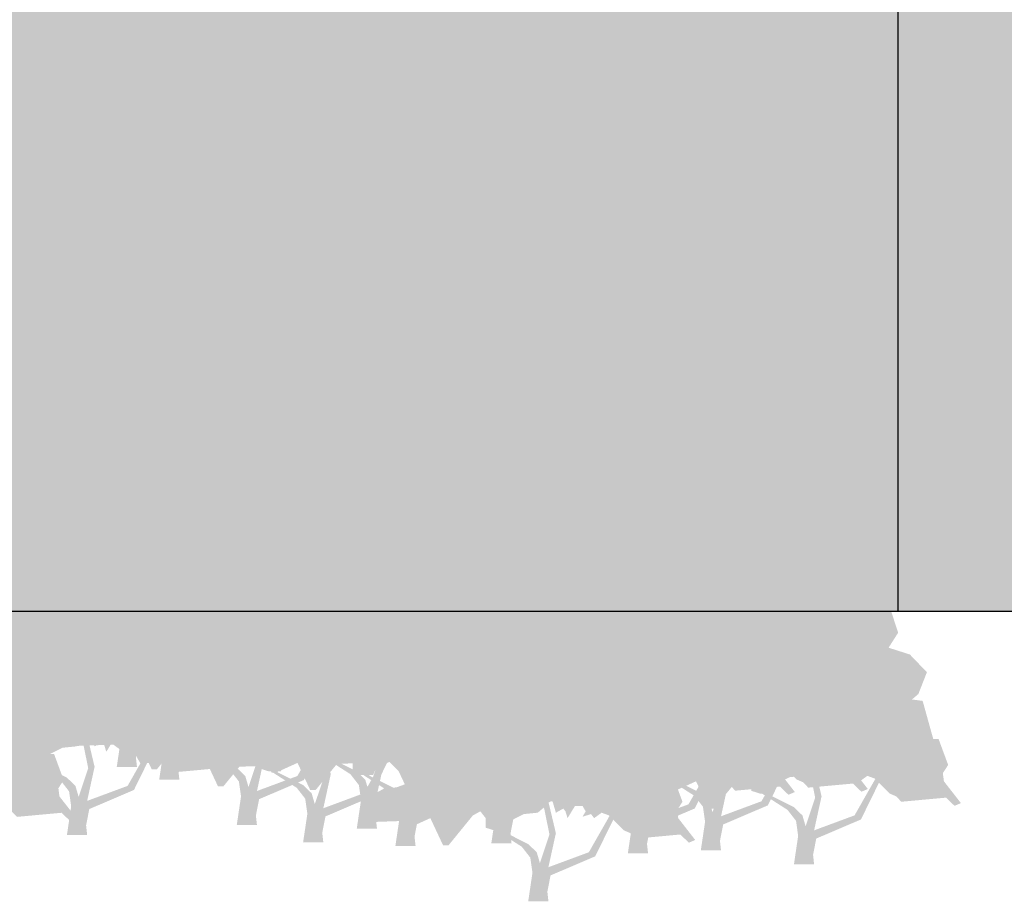
# Model space of a CAD drawing. Units: feet. Extents: x 2368 to 3224, y 836 to 1229.
# Tile 3 of 9: x 2413 to 2447, y 844 to 873. Entities that reach past the tile are written whole.
import ezdxf

# ---------------------------------------------------------------- set-up
doc = ezdxf.new("R2010")
doc.units = ezdxf.units.FT
for name, color, linetype, lineweight in [('A-ELEV', 7, 'Continuous', 25), ('A-ELEV-PATT', 8, 'Continuous', 13), ('L-PLNT', 3, 'Continuous', 13)]:
    doc.layers.add(name, color=color, linetype=linetype, lineweight=lineweight)

msp = doc.modelspace()

# ---------------------------------------------------------------- hatches: boundary and pattern name
at = {"layer": 'A-ELEV-PATT'}
h = msp.add_hatch(color=256, dxfattribs=at)
h.dxf.hatch_style = 1
h.paths.add_polyline_path([(2443.042, 973.51), (2394.909, 973.51), (2394.909, 853.51), (2443.042, 853.51)])
h.paths.add_polyline_path([(2422.205, 920.108), (2422.205, 905.784), (2416.403, 905.784), (2416.403, 920.108)], flags=16)
h.paths.add_polyline_path([(2449.299, 970.694), (2443.042, 973.51), (2443.042, 853.51), (2449.299, 853.51)])
h.paths.add_polyline_path([(2510.022, 987.861), (2368.302, 987.861), (2394.909, 973.51), (2443.042, 973.51), (2510.022, 973.51)])
h.paths.add_polyline_path([(2510.022, 973.51), (2443.042, 973.51), (2449.299, 970.694), (2510.022, 970.694)])
at = {"layer": 'L-PLNT'}
h = msp.add_hatch(color=256, dxfattribs=at)
h.dxf.hatch_style = 1
h.paths.add_polyline_path([(2428.131, 855.842), (2427.556, 856.441), (2426.837, 856.672), (2427.161, 857.179), (2426.873, 858.054), (2426.694, 858.054), (2426.334, 858.838), (2426.119, 858.791), (2425.867, 858.791), (2425.687, 859.16), (2425.795, 859.667), (2426.083, 859.667), (2425.543, 860.312), (2425.471, 860.824), (2425.184, 861.142), (2424.932, 860.865), (2424.789, 860.957), (2424.753, 861.188), (2424.573, 861.28), (2424.321, 861.049), (2424.034, 861.096), (2423.818, 860.681), (2423.818, 860.312), (2424.106, 860.174), (2423.89, 860.036), (2423.674, 860.22), (2423.063, 859.621), (2423.063, 859.483), (2422.812, 859.344), (2422.883, 859.206), (2423.063, 858.93), (2422.74, 858.699), (2422.416, 858.93), (2422.236, 858.884), (2422.165, 858.699), (2422.416, 858.653), (2422.452, 858.285), (2422.171, 858.331), (2421.841, 858.008), (2422.201, 857.962), (2422.057, 857.501), (2421.733, 857.455), (2421.374, 857.225), (2420.942, 856.994), (2420.907, 857.179), (2420.583, 856.487), (2421.158, 856.626), (2421.518, 856.395), (2421.41, 855.842), (2420.763, 855.612), (2420.475, 855.796), (2420.367, 855.52), (2420.116, 855.474), (2419.9, 855.197), (2419.648, 854.875), (2419.972, 854.598), (2420.188, 854.736), (2419.944, 854.336), (2420.121, 854.356), (2420.095, 853.994), (2419.505, 853.216), (2418.786, 853.17), (2418.462, 852.985), (2417.923, 852.386), (2418.139, 852.017), (2419.469, 852.064), (2419.72, 851.879), (2420.331, 852.156), (2420.763, 851.234), (2420.942, 851.234), (2421.769, 852.248), (2422.021, 852.386), (2422.201, 852.156), (2422.201, 851.833), (2422.488, 851.741), (2422.883, 851.741), (2423.027, 852.064), (2423.495, 852.294), (2423.962, 852.34), (2424.178, 852.524), (2424.213, 852.57), (2424.321, 852.801), (2424.465, 852.709), (2424.573, 852.34), (2424.825, 852.478), (2424.896, 852.386), (2424.968, 852.156), (2425.22, 852.57), (2425.472, 852.57), (2425.579, 852.386), (2425.472, 852.202), (2425.759, 852.294), (2425.867, 852.156), (2426.119, 852.34), (2426.37, 852.248), (2426.873, 851.741), (2427.089, 851.649), (2427.269, 851.465), (2428.778, 851.603), (2429.066, 851.326), (2429.282, 851.418), (2428.707, 852.156), (2428.671, 852.432), (2428.85, 852.709), (2428.527, 853.584), (2428.347, 853.584), (2427.988, 854.875), (2427.628, 854.921), (2427.844, 855.105)])
h = msp.add_hatch(color=256, dxfattribs=at)
h.dxf.hatch_style = 1
h.paths.add_polyline_path([(2414.456, 854.681), (2413.881, 855.281), (2413.162, 855.511), (2413.485, 856.018), (2413.198, 856.893), (2413.018, 856.893), (2412.659, 857.677), (2412.443, 857.631), (2412.191, 857.631), (2412.012, 857.999), (2412.12, 858.506), (2412.407, 858.506), (2411.868, 859.151), (2411.795, 859.663), (2411.509, 859.981), (2411.257, 859.704), (2411.113, 859.797), (2411.077, 860.027), (2410.897, 860.119), (2410.646, 859.889), (2410.358, 859.935), (2410.143, 859.52), (2410.143, 859.151), (2410.43, 859.013), (2410.214, 858.875), (2409.999, 859.059), (2409.388, 858.46), (2409.388, 858.322), (2409.136, 858.184), (2409.208, 858.045), (2409.388, 857.769), (2409.064, 857.539), (2408.741, 857.769), (2408.561, 857.723), (2408.489, 857.539), (2408.741, 857.492), (2408.777, 857.124), (2408.496, 857.17), (2408.166, 856.847), (2408.525, 856.801), (2408.381, 856.34), (2408.058, 856.294), (2407.698, 856.064), (2407.267, 855.834), (2407.231, 856.018), (2406.908, 855.327), (2407.483, 855.465), (2407.842, 855.234), (2407.734, 854.681), (2407.087, 854.451), (2406.8, 854.635), (2406.692, 854.359), (2406.44, 854.313), (2406.225, 854.036), (2405.973, 853.714), (2406.297, 853.437), (2406.512, 853.576), (2406.268, 853.175), (2406.445, 853.195), (2406.42, 852.833), (2405.829, 852.055), (2405.11, 852.009), (2404.787, 851.824), (2404.248, 851.225), (2404.463, 850.857), (2405.793, 850.903), (2406.045, 850.718), (2406.656, 850.995), (2407.087, 850.073), (2407.267, 850.073), (2408.094, 851.087), (2408.345, 851.225), (2408.525, 850.995), (2408.525, 850.672), (2408.813, 850.58), (2409.208, 850.58), (2409.352, 850.903), (2409.819, 851.133), (2410.286, 851.179), (2410.502, 851.364), (2410.538, 851.41), (2410.646, 851.64), (2410.79, 851.548), (2410.897, 851.179), (2411.149, 851.318), (2411.221, 851.225), (2411.293, 850.995), (2411.544, 851.41), (2411.796, 851.41), (2411.904, 851.225), (2411.796, 851.041), (2412.084, 851.133), (2412.191, 850.995), (2412.443, 851.179), (2412.695, 851.087), (2413.198, 850.58), (2413.414, 850.488), (2413.593, 850.304), (2415.103, 850.442), (2415.391, 850.165), (2415.606, 850.258), (2415.031, 850.995), (2414.995, 851.271), (2415.175, 851.548), (2414.851, 852.423), (2414.672, 852.423), (2414.312, 853.714), (2413.953, 853.76), (2414.168, 853.944)])
h = msp.add_hatch(color=256, dxfattribs=at)
h.dxf.hatch_style = 1
h.paths.add_polyline_path([(2421.127, 854.737), (2420.552, 855.336), (2419.833, 855.567), (2420.157, 856.074), (2419.869, 856.949), (2419.689, 856.949), (2419.33, 857.732), (2419.114, 857.686), (2418.862, 857.686), (2418.683, 858.055), (2418.791, 858.562), (2419.078, 858.562), (2418.539, 859.207), (2418.466, 859.718), (2418.18, 860.037), (2417.928, 859.76), (2417.784, 859.852), (2417.748, 860.083), (2417.568, 860.175), (2417.317, 859.944), (2417.029, 859.99), (2416.814, 859.576), (2416.814, 859.207), (2417.101, 859.069), (2416.886, 858.931), (2416.67, 859.115), (2416.059, 858.516), (2416.059, 858.378), (2415.807, 858.239), (2415.879, 858.101), (2416.059, 857.825), (2415.735, 857.594), (2415.412, 857.825), (2415.232, 857.779), (2415.16, 857.594), (2415.412, 857.548), (2415.448, 857.179), (2415.167, 857.226), (2414.837, 856.903), (2415.196, 856.857), (2415.052, 856.396), (2414.729, 856.35), (2414.369, 856.12), (2413.938, 855.889), (2413.902, 856.074), (2413.579, 855.382), (2414.154, 855.521), (2414.513, 855.29), (2414.405, 854.737), (2413.758, 854.507), (2413.471, 854.691), (2413.363, 854.415), (2413.111, 854.369), (2412.896, 854.092), (2412.644, 853.769), (2412.968, 853.493), (2413.183, 853.631), (2412.939, 853.23), (2413.117, 853.251), (2413.091, 852.888), (2412.5, 852.111), (2411.781, 852.064), (2411.458, 851.88), (2410.919, 851.281), (2411.134, 850.912), (2412.464, 850.958), (2412.716, 850.774), (2413.327, 851.051), (2413.758, 850.129), (2413.938, 850.129), (2414.765, 851.143), (2415.016, 851.281), (2415.196, 851.051), (2415.196, 850.728), (2415.484, 850.636), (2415.879, 850.636), (2416.023, 850.958), (2416.49, 851.189), (2416.957, 851.235), (2417.173, 851.419), (2417.209, 851.465), (2417.317, 851.696), (2417.461, 851.604), (2417.568, 851.235), (2417.82, 851.373), (2417.892, 851.281), (2417.964, 851.051), (2418.215, 851.465), (2418.467, 851.465), (2418.575, 851.281), (2418.467, 851.097), (2418.755, 851.189), (2418.862, 851.051), (2419.114, 851.235), (2419.366, 851.143), (2419.869, 850.636), (2420.085, 850.544), (2420.264, 850.359), (2421.774, 850.498), (2422.062, 850.221), (2422.277, 850.313), (2421.702, 851.051), (2421.666, 851.327), (2421.846, 851.604), (2421.522, 852.479), (2421.343, 852.479), (2420.983, 853.769), (2420.624, 853.816), (2420.839, 854)])
h = msp.add_hatch(color=256, dxfattribs=at)
h.dxf.hatch_style = 1
h.paths.add_polyline_path([(2422.561, 854.308), (2421.986, 854.907), (2421.267, 855.137), (2421.591, 855.644), (2421.303, 856.52), (2421.123, 856.52), (2420.764, 857.303), (2420.548, 857.257), (2420.297, 857.257), (2420.117, 857.626), (2420.225, 858.132), (2420.512, 858.132), (2419.973, 858.778), (2419.901, 859.289), (2419.614, 859.607), (2419.362, 859.331), (2419.218, 859.423), (2419.182, 859.653), (2419.003, 859.745), (2418.751, 859.515), (2418.463, 859.561), (2418.248, 859.146), (2418.248, 858.778), (2418.535, 858.639), (2418.32, 858.501), (2418.104, 858.685), (2417.493, 858.086), (2417.493, 857.948), (2417.241, 857.81), (2417.313, 857.672), (2417.493, 857.395), (2417.169, 857.165), (2416.846, 857.395), (2416.666, 857.349), (2416.594, 857.165), (2416.846, 857.119), (2416.882, 856.75), (2416.601, 856.796), (2416.271, 856.474), (2416.63, 856.427), (2416.486, 855.967), (2416.163, 855.921), (2415.804, 855.69), (2415.372, 855.46), (2415.336, 855.644), (2415.013, 854.953), (2415.588, 855.091), (2415.947, 854.861), (2415.839, 854.308), (2415.192, 854.077), (2414.905, 854.262), (2414.797, 853.985), (2414.545, 853.939), (2414.33, 853.663), (2414.078, 853.34), (2414.402, 853.063), (2414.617, 853.202), (2414.374, 852.801), (2414.551, 852.822), (2414.525, 852.459), (2413.934, 851.681), (2413.215, 851.635), (2412.892, 851.451), (2412.353, 850.852), (2412.568, 850.483), (2413.898, 850.529), (2414.15, 850.345), (2414.761, 850.621), (2415.192, 849.7), (2415.372, 849.7), (2416.199, 850.713), (2416.451, 850.852), (2416.63, 850.621), (2416.63, 850.299), (2416.918, 850.206), (2417.313, 850.206), (2417.457, 850.529), (2417.924, 850.759), (2418.392, 850.806), (2418.607, 850.99), (2418.643, 851.036), (2418.751, 851.266), (2418.895, 851.174), (2419.003, 850.806), (2419.254, 850.944), (2419.326, 850.852), (2419.398, 850.621), (2419.65, 851.036), (2419.901, 851.036), (2420.009, 850.852), (2419.901, 850.667), (2420.189, 850.759), (2420.297, 850.621), (2420.548, 850.806), (2420.8, 850.713), (2421.303, 850.206), (2421.519, 850.114), (2421.698, 849.93), (2423.208, 850.068), (2423.496, 849.792), (2423.711, 849.884), (2423.136, 850.621), (2423.1, 850.898), (2423.28, 851.174), (2422.957, 852.05), (2422.777, 852.05), (2422.417, 853.34), (2422.058, 853.386), (2422.274, 853.57)])
h = msp.add_hatch(color=256, dxfattribs=at)
h.dxf.hatch_style = 1
h.paths.add_polyline_path([(2425.182, 852.773), (2424.607, 853.372), (2423.888, 853.602), (2424.212, 854.109), (2423.924, 854.985), (2423.744, 854.985), (2423.385, 855.768), (2423.169, 855.722), (2422.918, 855.722), (2422.738, 856.09), (2422.846, 856.597), (2423.133, 856.597), (2422.594, 857.242), (2422.522, 857.754), (2422.235, 858.072), (2421.983, 857.795), (2421.839, 857.888), (2421.803, 858.118), (2421.624, 858.21), (2421.372, 857.98), (2421.085, 858.026), (2420.869, 857.611), (2420.869, 857.242), (2421.156, 857.104), (2420.941, 856.966), (2420.725, 857.15), (2420.114, 856.551), (2420.114, 856.413), (2419.862, 856.275), (2419.934, 856.137), (2420.114, 855.86), (2419.79, 855.63), (2419.467, 855.86), (2419.287, 855.814), (2419.215, 855.63), (2419.467, 855.584), (2419.503, 855.215), (2419.222, 855.261), (2418.892, 854.938), (2419.251, 854.892), (2419.108, 854.432), (2418.784, 854.385), (2418.425, 854.155), (2417.993, 853.925), (2417.957, 854.109), (2417.634, 853.418), (2418.209, 853.556), (2418.568, 853.326), (2418.461, 852.773), (2417.814, 852.542), (2417.526, 852.727), (2417.418, 852.45), (2417.167, 852.404), (2416.951, 852.127), (2416.699, 851.805), (2417.023, 851.528), (2417.238, 851.667), (2416.995, 851.266), (2417.172, 851.287), (2417.146, 850.924), (2416.555, 850.146), (2415.837, 850.1), (2415.513, 849.916), (2414.974, 849.316), (2415.19, 848.948), (2416.52, 848.994), (2416.771, 848.81), (2417.382, 849.086), (2417.814, 848.164), (2417.993, 848.164), (2418.82, 849.178), (2419.072, 849.316), (2419.251, 849.086), (2419.251, 848.763), (2419.539, 848.671), (2419.934, 848.671), (2420.078, 848.994), (2420.545, 849.224), (2421.013, 849.27), (2421.228, 849.455), (2421.264, 849.501), (2421.372, 849.731), (2421.516, 849.639), (2421.624, 849.27), (2421.875, 849.409), (2421.947, 849.316), (2422.019, 849.086), (2422.271, 849.501), (2422.522, 849.501), (2422.63, 849.316), (2422.522, 849.132), (2422.81, 849.224), (2422.918, 849.086), (2423.169, 849.27), (2423.421, 849.178), (2423.924, 848.671), (2424.14, 848.579), (2424.32, 848.395), (2425.829, 848.533), (2426.117, 848.257), (2426.332, 848.349), (2425.757, 849.086), (2425.721, 849.363), (2425.901, 849.639), (2425.578, 850.515), (2425.398, 850.515), (2425.038, 851.805), (2424.679, 851.851), (2424.895, 852.035)])
h = msp.add_hatch(color=256, dxfattribs=at)
h.dxf.hatch_style = 1
h.paths.add_polyline_path([(2429.237, 852.65), (2428.662, 853.249), (2427.943, 853.479), (2428.267, 853.986), (2427.979, 854.862), (2427.8, 854.862), (2427.44, 855.645), (2427.224, 855.599), (2426.973, 855.599), (2426.793, 855.968), (2426.901, 856.475), (2427.189, 856.475), (2426.649, 857.12), (2426.577, 857.631), (2426.29, 857.949), (2426.038, 857.673), (2425.895, 857.765), (2425.859, 857.995), (2425.679, 858.087), (2425.427, 857.857), (2425.14, 857.903), (2424.924, 857.488), (2424.924, 857.12), (2425.212, 856.981), (2424.996, 856.843), (2424.78, 857.028), (2424.169, 856.428), (2424.169, 856.29), (2423.918, 856.152), (2423.989, 856.014), (2424.169, 855.737), (2423.846, 855.507), (2423.522, 855.737), (2423.342, 855.691), (2423.271, 855.507), (2423.522, 855.461), (2423.558, 855.092), (2423.277, 855.138), (2422.947, 854.816), (2423.307, 854.77), (2423.163, 854.309), (2422.839, 854.263), (2422.48, 854.032), (2422.048, 853.802), (2422.012, 853.986), (2421.689, 853.295), (2422.264, 853.433), (2422.624, 853.203), (2422.516, 852.65), (2421.869, 852.419), (2421.581, 852.604), (2421.473, 852.327), (2421.222, 852.281), (2421.006, 852.005), (2420.754, 851.682), (2421.078, 851.406), (2421.294, 851.544), (2421.05, 851.143), (2421.227, 851.164), (2421.201, 850.801), (2420.611, 850.023), (2419.892, 849.977), (2419.568, 849.793), (2419.029, 849.194), (2419.245, 848.825), (2420.575, 848.871), (2420.826, 848.687), (2421.437, 848.963), (2421.869, 848.042), (2422.048, 848.042), (2422.875, 849.055), (2423.127, 849.194), (2423.307, 848.963), (2423.307, 848.641), (2423.594, 848.549), (2423.989, 848.549), (2424.133, 848.871), (2424.601, 849.102), (2425.068, 849.148), (2425.283, 849.332), (2425.319, 849.378), (2425.427, 849.608), (2425.571, 849.516), (2425.679, 849.148), (2425.93, 849.286), (2426.002, 849.194), (2426.074, 848.963), (2426.326, 849.378), (2426.577, 849.378), (2426.685, 849.194), (2426.577, 849.009), (2426.865, 849.102), (2426.973, 848.963), (2427.224, 849.148), (2427.476, 849.055), (2427.979, 848.549), (2428.195, 848.456), (2428.375, 848.272), (2429.884, 848.41), (2430.172, 848.134), (2430.388, 848.226), (2429.813, 848.963), (2429.777, 849.24), (2429.956, 849.516), (2429.633, 850.392), (2429.453, 850.392), (2429.094, 851.682), (2428.734, 851.728), (2428.95, 851.912)])
h = msp.add_hatch(color=256, dxfattribs=at)
h.dxf.hatch_style = 1
h.paths.add_polyline_path([(2419.444, 852.439), (2418.869, 853.038), (2418.15, 853.268), (2418.473, 853.775), (2418.186, 854.651), (2418.006, 854.651), (2417.647, 855.434), (2417.431, 855.388), (2417.179, 855.388), (2417, 855.757), (2417.107, 856.264), (2417.395, 856.264), (2416.856, 856.909), (2416.783, 857.42), (2416.496, 857.738), (2416.245, 857.462), (2416.101, 857.554), (2416.065, 857.784), (2415.885, 857.876), (2415.634, 857.646), (2415.346, 857.692), (2415.13, 857.277), (2415.13, 856.909), (2415.418, 856.77), (2415.202, 856.632), (2414.987, 856.817), (2414.376, 856.217), (2414.376, 856.079), (2414.124, 855.941), (2414.196, 855.803), (2414.376, 855.526), (2414.052, 855.296), (2413.729, 855.526), (2413.549, 855.48), (2413.477, 855.296), (2413.729, 855.25), (2413.764, 854.881), (2413.483, 854.927), (2413.153, 854.605), (2413.513, 854.559), (2413.369, 854.098), (2413.046, 854.052), (2412.686, 853.821), (2412.255, 853.591), (2412.219, 853.775), (2411.895, 853.084), (2412.47, 853.222), (2412.83, 852.992), (2412.722, 852.439), (2412.075, 852.208), (2411.788, 852.393), (2411.68, 852.116), (2411.428, 852.07), (2411.212, 851.794), (2410.961, 851.471), (2411.284, 851.195), (2411.5, 851.333), (2411.256, 850.932), (2411.433, 850.953), (2411.408, 850.59), (2410.817, 849.812), (2410.098, 849.766), (2409.775, 849.582), (2409.235, 848.983), (2409.451, 848.614), (2410.781, 848.66), (2411.033, 848.476), (2411.644, 848.752), (2412.075, 847.831), (2412.255, 847.831), (2413.082, 848.844), (2413.333, 848.983), (2413.513, 848.752), (2413.513, 848.43), (2413.8, 848.338), (2414.196, 848.338), (2414.34, 848.66), (2414.807, 848.89), (2415.274, 848.937), (2415.49, 849.121), (2415.526, 849.167), (2415.634, 849.397), (2415.777, 849.305), (2415.885, 848.937), (2416.137, 849.075), (2416.209, 848.983), (2416.281, 848.752), (2416.532, 849.167), (2416.784, 849.167), (2416.892, 848.983), (2416.784, 848.798), (2417.071, 848.89), (2417.179, 848.752), (2417.431, 848.937), (2417.682, 848.844), (2418.186, 848.338), (2418.401, 848.245), (2418.581, 848.061), (2420.091, 848.199), (2420.378, 847.923), (2420.594, 848.015), (2420.019, 848.752), (2419.983, 849.029), (2420.163, 849.305), (2419.839, 850.181), (2419.659, 850.181), (2419.3, 851.471), (2418.941, 851.517), (2419.156, 851.701)])
h = msp.add_hatch(color=256, dxfattribs=at)
h.dxf.hatch_style = 1
h.paths.add_polyline_path([(2427.424, 852.19), (2426.849, 852.789), (2426.13, 853.019), (2426.454, 853.526), (2426.166, 854.401), (2425.986, 854.401), (2425.627, 855.185), (2425.411, 855.139), (2425.16, 855.139), (2424.98, 855.507), (2425.088, 856.014), (2425.375, 856.014), (2424.836, 856.659), (2424.764, 857.171), (2424.477, 857.489), (2424.225, 857.212), (2424.081, 857.305), (2424.045, 857.535), (2423.866, 857.627), (2423.614, 857.397), (2423.327, 857.443), (2423.111, 857.028), (2423.111, 856.659), (2423.398, 856.521), (2423.183, 856.383), (2422.967, 856.567), (2422.356, 855.968), (2422.356, 855.83), (2422.104, 855.692), (2422.176, 855.554), (2422.356, 855.277), (2422.033, 855.047), (2421.709, 855.277), (2421.529, 855.231), (2421.457, 855.047), (2421.709, 855.001), (2421.745, 854.632), (2421.464, 854.678), (2421.134, 854.355), (2421.493, 854.309), (2421.35, 853.849), (2421.026, 853.802), (2420.667, 853.572), (2420.235, 853.342), (2420.199, 853.526), (2419.876, 852.835), (2420.451, 852.973), (2420.81, 852.743), (2420.703, 852.19), (2420.056, 851.959), (2419.768, 852.143), (2419.66, 851.867), (2419.409, 851.821), (2419.193, 851.544), (2418.941, 851.222), (2419.265, 850.945), (2419.48, 851.084), (2419.237, 850.683), (2419.414, 850.704), (2419.388, 850.341), (2418.797, 849.563), (2418.079, 849.517), (2417.755, 849.333), (2417.216, 848.733), (2417.432, 848.365), (2418.762, 848.411), (2419.013, 848.227), (2419.624, 848.503), (2420.056, 847.581), (2420.235, 847.581), (2421.062, 848.595), (2421.314, 848.733), (2421.493, 848.503), (2421.493, 848.18), (2421.781, 848.088), (2422.176, 848.088), (2422.32, 848.411), (2422.787, 848.641), (2423.255, 848.687), (2423.47, 848.872), (2423.506, 848.918), (2423.614, 849.148), (2423.758, 849.056), (2423.866, 848.687), (2424.117, 848.826), (2424.189, 848.733), (2424.261, 848.503), (2424.513, 848.918), (2424.764, 848.918), (2424.872, 848.733), (2424.764, 848.549), (2425.052, 848.641), (2425.16, 848.503), (2425.411, 848.687), (2425.663, 848.595), (2426.166, 848.088), (2426.382, 847.996), (2426.562, 847.812), (2428.071, 847.95), (2428.359, 847.674), (2428.574, 847.766), (2427.999, 848.503), (2427.963, 848.78), (2428.143, 849.056), (2427.82, 849.932), (2427.64, 849.932), (2427.28, 851.222), (2426.921, 851.268), (2427.137, 851.452)])
h = msp.add_hatch(color=256, dxfattribs=at)
h.dxf.hatch_style = 1
h.paths.add_polyline_path([(2430.542, 852.065), (2429.966, 852.664), (2429.248, 852.894), (2429.571, 853.401), (2429.284, 854.277), (2429.104, 854.277), (2428.744, 855.06), (2428.529, 855.014), (2428.277, 855.014), (2428.097, 855.383), (2428.205, 855.89), (2428.493, 855.89), (2427.954, 856.535), (2427.881, 857.046), (2427.594, 857.364), (2427.343, 857.088), (2427.199, 857.18), (2427.163, 857.41), (2426.983, 857.503), (2426.731, 857.272), (2426.444, 857.318), (2426.228, 856.904), (2426.228, 856.535), (2426.516, 856.397), (2426.3, 856.258), (2426.084, 856.443), (2425.473, 855.844), (2425.473, 855.705), (2425.222, 855.567), (2425.294, 855.429), (2425.473, 855.152), (2425.15, 854.922), (2424.826, 855.152), (2424.647, 855.106), (2424.575, 854.922), (2424.826, 854.876), (2424.862, 854.507), (2424.581, 854.553), (2424.251, 854.231), (2424.611, 854.185), (2424.467, 853.724), (2424.143, 853.678), (2423.784, 853.447), (2423.353, 853.217), (2423.317, 853.401), (2422.993, 852.71), (2423.568, 852.848), (2423.928, 852.618), (2423.82, 852.065), (2423.173, 851.835), (2422.885, 852.019), (2422.778, 851.742), (2422.526, 851.696), (2422.31, 851.42), (2422.059, 851.097), (2422.382, 850.821), (2422.598, 850.959), (2422.354, 850.558), (2422.531, 850.579), (2422.506, 850.216), (2421.915, 849.438), (2421.196, 849.392), (2420.872, 849.208), (2420.333, 848.609), (2420.549, 848.24), (2421.879, 848.286), (2422.131, 848.102), (2422.742, 848.378), (2423.173, 847.457), (2423.353, 847.457), (2424.179, 848.471), (2424.431, 848.609), (2424.611, 848.378), (2424.611, 848.056), (2424.898, 847.964), (2425.294, 847.964), (2425.437, 848.286), (2425.905, 848.517), (2426.372, 848.563), (2426.588, 848.747), (2426.624, 848.793), (2426.731, 849.024), (2426.875, 848.931), (2426.983, 848.563), (2427.235, 848.701), (2427.307, 848.609), (2427.378, 848.378), (2427.63, 848.793), (2427.882, 848.793), (2427.99, 848.609), (2427.882, 848.425), (2428.169, 848.517), (2428.277, 848.378), (2428.529, 848.563), (2428.78, 848.471), (2429.284, 847.964), (2429.499, 847.872), (2429.679, 847.687), (2431.189, 847.825), (2431.476, 847.549), (2431.692, 847.641), (2431.117, 848.378), (2431.081, 848.655), (2431.261, 848.931), (2430.937, 849.807), (2430.757, 849.807), (2430.398, 851.097), (2430.038, 851.143), (2430.254, 851.328)])
h = msp.add_hatch(color=256, dxfattribs=at)
h.dxf.hatch_style = 1
h.paths.add_polyline_path([(2433.784, 852.159), (2433.209, 852.758), (2432.49, 852.988), (2432.814, 853.495), (2432.526, 854.371), (2432.346, 854.371), (2431.987, 855.154), (2431.771, 855.108), (2431.52, 855.108), (2431.34, 855.477), (2431.448, 855.983), (2431.735, 855.983), (2431.196, 856.629), (2431.124, 857.14), (2430.837, 857.458), (2430.585, 857.182), (2430.441, 857.274), (2430.405, 857.504), (2430.226, 857.596), (2429.974, 857.366), (2429.686, 857.412), (2429.471, 856.997), (2429.471, 856.629), (2429.758, 856.49), (2429.543, 856.352), (2429.327, 856.536), (2428.716, 855.937), (2428.716, 855.799), (2428.464, 855.661), (2428.536, 855.523), (2428.716, 855.246), (2428.392, 855.016), (2428.069, 855.246), (2427.889, 855.2), (2427.817, 855.016), (2428.069, 854.97), (2428.105, 854.601), (2427.824, 854.647), (2427.494, 854.324), (2427.853, 854.278), (2427.709, 853.818), (2427.386, 853.772), (2427.027, 853.541), (2426.595, 853.311), (2426.559, 853.495), (2426.236, 852.804), (2426.811, 852.942), (2427.17, 852.712), (2427.062, 852.159), (2426.415, 851.928), (2426.128, 852.113), (2426.02, 851.836), (2425.768, 851.79), (2425.553, 851.514), (2425.301, 851.191), (2425.625, 850.914), (2425.84, 851.053), (2425.596, 850.652), (2425.774, 850.673), (2425.748, 850.31), (2425.157, 849.532), (2424.438, 849.486), (2424.115, 849.302), (2423.576, 848.703), (2423.791, 848.334), (2425.121, 848.38), (2425.373, 848.196), (2425.984, 848.472), (2426.415, 847.551), (2426.595, 847.551), (2427.422, 848.564), (2427.674, 848.703), (2427.853, 848.472), (2427.853, 848.15), (2428.141, 848.057), (2428.536, 848.057), (2428.68, 848.38), (2429.147, 848.61), (2429.615, 848.656), (2429.83, 848.841), (2429.866, 848.887), (2429.974, 849.117), (2430.118, 849.025), (2430.226, 848.656), (2430.477, 848.795), (2430.549, 848.703), (2430.621, 848.472), (2430.873, 848.887), (2431.124, 848.887), (2431.232, 848.703), (2431.124, 848.518), (2431.412, 848.61), (2431.52, 848.472), (2431.771, 848.656), (2432.023, 848.564), (2432.526, 848.057), (2432.742, 847.965), (2432.921, 847.781), (2434.431, 847.919), (2434.719, 847.643), (2434.934, 847.735), (2434.359, 848.472), (2434.323, 848.749), (2434.503, 849.025), (2434.18, 849.901), (2434, 849.901), (2433.64, 851.191), (2433.281, 851.237), (2433.497, 851.421)])
h = msp.add_hatch(color=256, dxfattribs=at)
h.dxf.hatch_style = 1
h.paths.add_polyline_path([(2438.397, 851.816), (2437.822, 852.415), (2437.103, 852.645), (2437.427, 853.152), (2437.139, 854.028), (2436.96, 854.028), (2436.6, 854.811), (2436.384, 854.765), (2436.133, 854.765), (2435.953, 855.134), (2436.061, 855.641), (2436.349, 855.641), (2435.809, 856.286), (2435.737, 856.797), (2435.45, 857.115), (2435.198, 856.839), (2435.055, 856.931), (2435.019, 857.161), (2434.839, 857.253), (2434.587, 857.023), (2434.3, 857.069), (2434.084, 856.654), (2434.084, 856.286), (2434.372, 856.147), (2434.156, 856.009), (2433.94, 856.194), (2433.329, 855.594), (2433.329, 855.456), (2433.078, 855.318), (2433.149, 855.18), (2433.329, 854.903), (2433.006, 854.673), (2432.682, 854.903), (2432.502, 854.857), (2432.431, 854.673), (2432.682, 854.627), (2432.718, 854.258), (2432.437, 854.304), (2432.107, 853.982), (2432.466, 853.936), (2432.323, 853.475), (2431.999, 853.429), (2431.64, 853.198), (2431.208, 852.968), (2431.172, 853.152), (2430.849, 852.461), (2431.424, 852.599), (2431.784, 852.369), (2431.676, 851.816), (2431.029, 851.585), (2430.741, 851.77), (2430.633, 851.493), (2430.382, 851.447), (2430.166, 851.171), (2429.914, 850.848), (2430.238, 850.572), (2430.454, 850.71), (2430.21, 850.309), (2430.387, 850.33), (2430.361, 849.967), (2429.771, 849.189), (2429.052, 849.143), (2428.728, 848.959), (2428.189, 848.36), (2428.405, 847.991), (2429.735, 848.037), (2429.986, 847.853), (2430.597, 848.129), (2431.029, 847.208), (2431.208, 847.208), (2432.035, 848.221), (2432.287, 848.36), (2432.466, 848.129), (2432.466, 847.807), (2432.754, 847.715), (2433.149, 847.715), (2433.293, 848.037), (2433.761, 848.268), (2434.228, 848.314), (2434.443, 848.498), (2434.479, 848.544), (2434.587, 848.774), (2434.731, 848.682), (2434.839, 848.314), (2435.09, 848.452), (2435.162, 848.36), (2435.234, 848.129), (2435.486, 848.544), (2435.737, 848.544), (2435.845, 848.36), (2435.737, 848.175), (2436.025, 848.268), (2436.133, 848.129), (2436.384, 848.314), (2436.636, 848.221), (2437.139, 847.715), (2437.355, 847.622), (2437.535, 847.438), (2439.044, 847.576), (2439.332, 847.3), (2439.548, 847.392), (2438.973, 848.129), (2438.937, 848.406), (2439.116, 848.682), (2438.793, 849.558), (2438.613, 849.558), (2438.254, 850.848), (2437.894, 850.894), (2438.11, 851.078)])
h = msp.add_hatch(color=256, dxfattribs=at)
h.dxf.hatch_style = 1
h.paths.add_polyline_path([(2440.863, 851.918), (2440.288, 852.517), (2439.569, 852.748), (2439.893, 853.255), (2439.605, 854.13), (2439.425, 854.13), (2439.066, 854.914), (2438.85, 854.868), (2438.599, 854.868), (2438.419, 855.236), (2438.527, 855.743), (2438.814, 855.743), (2438.275, 856.388), (2438.203, 856.9), (2437.916, 857.218), (2437.664, 856.941), (2437.52, 857.033), (2437.484, 857.264), (2437.305, 857.356), (2437.053, 857.126), (2436.766, 857.172), (2436.55, 856.757), (2436.55, 856.388), (2436.837, 856.25), (2436.622, 856.112), (2436.406, 856.296), (2435.795, 855.697), (2435.795, 855.559), (2435.543, 855.421), (2435.615, 855.282), (2435.795, 855.006), (2435.472, 854.775), (2435.148, 855.006), (2434.968, 854.96), (2434.896, 854.775), (2435.148, 854.729), (2435.184, 854.361), (2434.903, 854.407), (2434.573, 854.084), (2434.932, 854.038), (2434.789, 853.577), (2434.465, 853.531), (2434.106, 853.301), (2433.674, 853.07), (2433.638, 853.255), (2433.315, 852.564), (2433.89, 852.702), (2434.249, 852.471), (2434.142, 851.918), (2433.495, 851.688), (2433.207, 851.872), (2433.099, 851.596), (2432.848, 851.55), (2432.632, 851.273), (2432.38, 850.951), (2432.704, 850.674), (2432.919, 850.812), (2432.676, 850.412), (2432.853, 850.432), (2432.827, 850.07), (2432.237, 849.292), (2431.518, 849.246), (2431.194, 849.061), (2430.655, 848.462), (2430.871, 848.094), (2432.201, 848.14), (2432.452, 847.955), (2433.063, 848.232), (2433.495, 847.31), (2433.674, 847.31), (2434.501, 848.324), (2434.753, 848.462), (2434.932, 848.232), (2434.932, 847.909), (2435.22, 847.817), (2435.615, 847.817), (2435.759, 848.14), (2436.226, 848.37), (2436.694, 848.416), (2436.909, 848.601), (2436.945, 848.647), (2437.053, 848.877), (2437.197, 848.785), (2437.305, 848.416), (2437.556, 848.554), (2437.628, 848.462), (2437.7, 848.232), (2437.952, 848.647), (2438.203, 848.647), (2438.311, 848.462), (2438.203, 848.278), (2438.491, 848.37), (2438.599, 848.232), (2438.85, 848.416), (2439.102, 848.324), (2439.605, 847.817), (2439.821, 847.725), (2440.001, 847.541), (2441.51, 847.679), (2441.798, 847.402), (2442.014, 847.495), (2441.438, 848.232), (2441.402, 848.508), (2441.582, 848.785), (2441.259, 849.66), (2441.079, 849.66), (2440.719, 850.951), (2440.36, 850.997), (2440.576, 851.181)])
h = msp.add_hatch(color=256, dxfattribs=at)
h.dxf.hatch_style = 1
h.paths.add_polyline_path([(2444.009, 851.442), (2443.434, 852.041), (2442.715, 852.271), (2443.038, 852.778), (2442.751, 853.654), (2442.571, 853.654), (2442.211, 854.437), (2441.996, 854.391), (2441.744, 854.391), (2441.564, 854.76), (2441.672, 855.267), (2441.96, 855.267), (2441.421, 855.912), (2441.348, 856.423), (2441.061, 856.741), (2440.81, 856.465), (2440.666, 856.557), (2440.63, 856.787), (2440.45, 856.88), (2440.198, 856.649), (2439.911, 856.695), (2439.695, 856.281), (2439.695, 855.912), (2439.983, 855.774), (2439.767, 855.635), (2439.551, 855.82), (2438.94, 855.221), (2438.94, 855.082), (2438.689, 854.944), (2438.761, 854.806), (2438.94, 854.529), (2438.617, 854.299), (2438.293, 854.529), (2438.114, 854.483), (2438.042, 854.299), (2438.293, 854.253), (2438.329, 853.884), (2438.048, 853.93), (2437.718, 853.608), (2438.078, 853.562), (2437.934, 853.101), (2437.61, 853.055), (2437.251, 852.824), (2436.82, 852.594), (2436.784, 852.778), (2436.46, 852.087), (2437.035, 852.225), (2437.395, 851.995), (2437.287, 851.442), (2436.64, 851.212), (2436.352, 851.396), (2436.245, 851.119), (2435.993, 851.073), (2435.777, 850.797), (2435.526, 850.474), (2435.849, 850.198), (2436.065, 850.336), (2435.821, 849.935), (2435.998, 849.956), (2435.973, 849.593), (2435.382, 848.815), (2434.663, 848.769), (2434.339, 848.585), (2433.8, 847.986), (2434.016, 847.617), (2435.346, 847.663), (2435.598, 847.479), (2436.209, 847.755), (2436.64, 846.834), (2436.82, 846.834), (2437.646, 847.848), (2437.898, 847.986), (2438.078, 847.755), (2438.078, 847.433), (2438.365, 847.341), (2438.761, 847.341), (2438.904, 847.663), (2439.372, 847.894), (2439.839, 847.94), (2440.055, 848.124), (2440.091, 848.17), (2440.198, 848.401), (2440.342, 848.308), (2440.45, 847.94), (2440.702, 848.078), (2440.774, 847.986), (2440.845, 847.755), (2441.097, 848.17), (2441.349, 848.17), (2441.457, 847.986), (2441.349, 847.802), (2441.636, 847.894), (2441.744, 847.755), (2441.996, 847.94), (2442.247, 847.848), (2442.751, 847.341), (2442.966, 847.249), (2443.146, 847.064), (2444.656, 847.203), (2444.943, 846.926), (2445.159, 847.018), (2444.584, 847.755), (2444.548, 848.032), (2444.728, 848.308), (2444.404, 849.184), (2444.224, 849.184), (2443.865, 850.474), (2443.505, 850.52), (2443.721, 850.705)])
h = msp.add_hatch(color=256, dxfattribs=at)
h.dxf.hatch_style = 1
h.paths.add_polyline_path([(2414.123, 850.931), (2413.547, 851.53), (2412.829, 851.76), (2413.152, 852.267), (2412.865, 853.143), (2412.685, 853.143), (2412.325, 853.926), (2412.11, 853.88), (2411.858, 853.88), (2411.678, 854.249), (2411.786, 854.756), (2412.074, 854.756), (2411.535, 855.401), (2411.462, 855.912), (2411.175, 856.23), (2410.924, 855.954), (2410.78, 856.046), (2410.744, 856.276), (2410.564, 856.368), (2410.312, 856.138), (2410.025, 856.184), (2409.809, 855.769), (2409.809, 855.401), (2410.097, 855.262), (2409.881, 855.124), (2409.665, 855.309), (2409.054, 854.709), (2409.054, 854.571), (2408.803, 854.433), (2408.875, 854.295), (2409.054, 854.018), (2408.731, 853.788), (2408.407, 854.018), (2408.228, 853.972), (2408.156, 853.788), (2408.407, 853.742), (2408.443, 853.373), (2408.162, 853.419), (2407.832, 853.097), (2408.192, 853.051), (2408.048, 852.59), (2407.724, 852.544), (2407.365, 852.313), (2406.934, 852.083), (2406.898, 852.267), (2406.574, 851.576), (2407.149, 851.714), (2407.509, 851.484), (2407.401, 850.931), (2406.754, 850.7), (2406.466, 850.885), (2406.359, 850.608), (2406.107, 850.562), (2405.891, 850.286), (2405.64, 849.963), (2405.963, 849.687), (2406.179, 849.825), (2405.935, 849.424), (2406.112, 849.445), (2406.086, 849.082), (2405.496, 848.304), (2404.777, 848.258), (2404.453, 848.074), (2403.914, 847.475), (2404.13, 847.106), (2405.46, 847.152), (2405.711, 846.968), (2406.323, 847.244), (2406.754, 846.323), (2406.934, 846.323), (2407.76, 847.336), (2408.012, 847.475), (2408.192, 847.244), (2408.192, 846.922), (2408.479, 846.83), (2408.875, 846.83), (2409.018, 847.152), (2409.486, 847.383), (2409.953, 847.429), (2410.169, 847.613), (2410.205, 847.659), (2410.312, 847.889), (2410.456, 847.797), (2410.564, 847.429), (2410.816, 847.567), (2410.888, 847.475), (2410.959, 847.244), (2411.211, 847.659), (2411.463, 847.659), (2411.571, 847.475), (2411.463, 847.29), (2411.75, 847.383), (2411.858, 847.244), (2412.11, 847.429), (2412.361, 847.336), (2412.865, 846.83), (2413.08, 846.737), (2413.26, 846.553), (2414.77, 846.691), (2415.057, 846.415), (2415.273, 846.507), (2414.698, 847.244), (2414.662, 847.521), (2414.841, 847.797), (2414.518, 848.673), (2414.338, 848.673), (2413.979, 849.963), (2413.619, 850.009), (2413.835, 850.193)])
h = msp.add_hatch(color=256, dxfattribs=at)
h.dxf.hatch_style = 1
h.paths.add_polyline_path([(2435.031, 850.196), (2434.456, 850.795), (2433.737, 851.026), (2434.06, 851.532), (2433.773, 852.408), (2433.593, 852.408), (2433.233, 853.191), (2433.018, 853.145), (2432.766, 853.145), (2432.586, 853.514), (2432.694, 854.021), (2432.982, 854.021), (2432.443, 854.666), (2432.37, 855.177), (2432.083, 855.495), (2431.832, 855.219), (2431.688, 855.311), (2431.652, 855.541), (2431.472, 855.634), (2431.22, 855.403), (2430.933, 855.449), (2430.717, 855.035), (2430.717, 854.666), (2431.005, 854.528), (2430.789, 854.389), (2430.573, 854.574), (2429.962, 853.975), (2429.962, 853.836), (2429.711, 853.698), (2429.783, 853.56), (2429.962, 853.284), (2429.639, 853.053), (2429.315, 853.284), (2429.136, 853.237), (2429.064, 853.053), (2429.315, 853.007), (2429.351, 852.638), (2429.07, 852.684), (2428.74, 852.362), (2429.1, 852.316), (2428.956, 851.855), (2428.632, 851.809), (2428.273, 851.578), (2427.842, 851.348), (2427.806, 851.532), (2427.482, 850.841), (2428.057, 850.979), (2428.417, 850.749), (2428.309, 850.196), (2427.662, 849.966), (2427.374, 850.15), (2427.267, 849.873), (2427.015, 849.827), (2426.799, 849.551), (2426.548, 849.228), (2426.871, 848.952), (2427.087, 849.09), (2426.843, 848.689), (2427.02, 848.71), (2426.995, 848.347), (2426.404, 847.569), (2425.685, 847.523), (2425.361, 847.339), (2424.822, 846.74), (2425.038, 846.371), (2426.368, 846.417), (2426.62, 846.233), (2427.231, 846.51), (2427.662, 845.588), (2427.842, 845.588), (2428.668, 846.602), (2428.92, 846.74), (2429.1, 846.51), (2429.1, 846.187), (2429.387, 846.095), (2429.783, 846.095), (2429.926, 846.417), (2430.394, 846.648), (2430.861, 846.694), (2431.077, 846.878), (2431.113, 846.924), (2431.22, 847.155), (2431.364, 847.063), (2431.472, 846.694), (2431.724, 846.832), (2431.796, 846.74), (2431.867, 846.51), (2432.119, 846.924), (2432.371, 846.924), (2432.479, 846.74), (2432.371, 846.556), (2432.658, 846.648), (2432.766, 846.51), (2433.018, 846.694), (2433.269, 846.602), (2433.773, 846.095), (2433.988, 846.003), (2434.168, 845.818), (2435.678, 845.957), (2435.965, 845.68), (2436.181, 845.772), (2435.606, 846.51), (2435.57, 846.786), (2435.75, 847.063), (2435.426, 847.938), (2435.246, 847.938), (2434.887, 849.228), (2434.527, 849.274), (2434.743, 849.459)])
h = msp.add_hatch(color=256, dxfattribs=at)
h.dxf.hatch_style = 1
h.paths.add_polyline_path([(2424.393, 850.22), (2425.903, 850.865), (2426.512, 852.105), (2426.387, 852.231), (2426.37, 852.202), (2425.687, 851.004), (2424.321, 850.497), (2424.573, 851.649), (2424.321, 852.709), (2424.307, 852.77), (2424.213, 852.57), (2424.178, 852.524), (2424.155, 852.505), (2424.178, 852.478), (2424.357, 851.603), (2424.034, 850.635), (2423.926, 851.004), (2423.638, 851.28), (2422.812, 851.695), (2422.741, 851.741), (2422.56, 851.741), (2423.423, 851.188), (2423.71, 850.819), (2423.782, 850.312), (2423.638, 849.345), (2424.321, 849.345), (2424.285, 849.667)])
h = msp.add_hatch(color=256, dxfattribs=at)
h.dxf.hatch_style = 1
h.paths.add_polyline_path([(2417.389, 849.115), (2418.898, 849.76), (2419.507, 851), (2419.382, 851.126), (2419.366, 851.097), (2418.683, 849.899), (2417.317, 849.392), (2417.568, 850.544), (2417.317, 851.604), (2417.302, 851.665), (2417.209, 851.465), (2417.173, 851.419), (2417.15, 851.4), (2417.173, 851.373), (2417.353, 850.498), (2417.029, 849.53), (2416.921, 849.899), (2416.634, 850.175), (2415.807, 850.59), (2415.736, 850.636), (2415.556, 850.636), (2416.418, 850.083), (2416.706, 849.714), (2416.778, 849.207), (2416.634, 848.24), (2417.317, 848.24), (2417.281, 848.562)])
h = msp.add_hatch(color=256, dxfattribs=at)
h.dxf.hatch_style = 1
h.paths.add_polyline_path([(2418.823, 848.686), (2420.333, 849.331), (2420.941, 850.571), (2420.817, 850.697), (2420.8, 850.667), (2420.117, 849.469), (2418.751, 848.962), (2419.003, 850.114), (2418.751, 851.174), (2418.736, 851.235), (2418.643, 851.036), (2418.607, 850.99), (2418.584, 850.97), (2418.607, 850.944), (2418.787, 850.068), (2418.463, 849.1), (2418.356, 849.469), (2418.068, 849.746), (2417.241, 850.16), (2417.171, 850.206), (2416.99, 850.206), (2417.852, 849.653), (2418.14, 849.285), (2418.212, 848.778), (2418.068, 847.81), (2418.751, 847.81), (2418.715, 848.133)])
h = msp.add_hatch(color=256, dxfattribs=at)
h.dxf.hatch_style = 1
h.paths.add_polyline_path([(2421.444, 847.151), (2422.954, 847.796), (2423.563, 849.036), (2423.438, 849.161), (2423.421, 849.132), (2422.738, 847.934), (2421.372, 847.427), (2421.624, 848.579), (2421.372, 849.639), (2421.358, 849.7), (2421.264, 849.501), (2421.228, 849.455), (2421.206, 849.435), (2421.228, 849.409), (2421.408, 848.533), (2421.085, 847.565), (2420.977, 847.934), (2420.689, 848.211), (2419.862, 848.625), (2419.792, 848.671), (2419.611, 848.671), (2420.473, 848.118), (2420.761, 847.75), (2420.833, 847.243), (2420.689, 846.275), (2421.372, 846.275), (2421.336, 846.598)])
h = msp.add_hatch(color=256, dxfattribs=at)
h.dxf.hatch_style = 1
h.paths.add_polyline_path([(2425.499, 847.028), (2427.009, 847.673), (2427.618, 848.913), (2427.493, 849.039), (2427.476, 849.009), (2426.793, 847.811), (2425.427, 847.304), (2425.679, 848.456), (2425.427, 849.516), (2425.413, 849.577), (2425.319, 849.378), (2425.283, 849.332), (2425.261, 849.312), (2425.283, 849.286), (2425.463, 848.41), (2425.14, 847.443), (2425.032, 847.811), (2424.744, 848.088), (2423.918, 848.502), (2423.847, 848.549), (2423.666, 848.549), (2424.529, 847.996), (2424.816, 847.627), (2424.888, 847.12), (2424.744, 846.152), (2425.427, 846.152), (2425.391, 846.475)])
h = msp.add_hatch(color=256, dxfattribs=at)
h.dxf.hatch_style = 1
h.paths.add_polyline_path([(2415.706, 846.817), (2417.215, 847.462), (2417.824, 848.702), (2417.699, 848.828), (2417.682, 848.798), (2417, 847.6), (2415.634, 847.093), (2415.885, 848.245), (2415.634, 849.305), (2415.619, 849.366), (2415.526, 849.167), (2415.49, 849.121), (2415.467, 849.101), (2415.49, 849.075), (2415.67, 848.199), (2415.346, 847.232), (2415.238, 847.6), (2414.951, 847.877), (2414.124, 848.291), (2414.053, 848.338), (2413.872, 848.338), (2414.735, 847.785), (2415.023, 847.416), (2415.094, 846.909), (2414.951, 845.941), (2415.634, 845.941), (2415.598, 846.264)])
h = msp.add_hatch(color=256, dxfattribs=at)
h.dxf.hatch_style = 1
h.paths.add_polyline_path([(2423.686, 846.568), (2425.196, 847.213), (2425.805, 848.453), (2425.68, 848.578), (2425.663, 848.549), (2424.98, 847.351), (2423.614, 846.844), (2423.866, 847.996), (2423.614, 849.056), (2423.6, 849.117), (2423.506, 848.918), (2423.47, 848.872), (2423.448, 848.852), (2423.47, 848.826), (2423.65, 847.95), (2423.327, 846.982), (2423.219, 847.351), (2422.931, 847.628), (2422.104, 848.042), (2422.034, 848.088), (2421.853, 848.088), (2422.715, 847.535), (2423.003, 847.167), (2423.075, 846.66), (2422.931, 845.692), (2423.614, 845.692), (2423.578, 846.015)])
h = msp.add_hatch(color=256, dxfattribs=at)
h.dxf.hatch_style = 1
h.paths.add_polyline_path([(2430.046, 846.537), (2431.556, 847.182), (2432.164, 848.422), (2432.04, 848.547), (2432.023, 848.518), (2431.34, 847.32), (2429.974, 846.813), (2430.226, 847.965), (2429.974, 849.025), (2429.959, 849.086), (2429.866, 848.887), (2429.83, 848.841), (2429.807, 848.821), (2429.83, 848.795), (2430.01, 847.919), (2429.686, 846.951), (2429.579, 847.32), (2429.291, 847.597), (2428.464, 848.011), (2428.394, 848.057), (2428.213, 848.057), (2429.075, 847.504), (2429.363, 847.136), (2429.435, 846.629), (2429.291, 845.661), (2429.974, 845.661), (2429.938, 845.984)])
h = msp.add_hatch(color=256, dxfattribs=at)
h.dxf.hatch_style = 1
h.paths.add_polyline_path([(2426.803, 846.443), (2428.313, 847.088), (2428.922, 848.328), (2428.797, 848.454), (2428.78, 848.425), (2428.097, 847.226), (2426.731, 846.72), (2426.983, 847.872), (2426.731, 848.931), (2426.717, 848.993), (2426.624, 848.793), (2426.588, 848.747), (2426.565, 848.728), (2426.588, 848.701), (2426.767, 847.825), (2426.444, 846.858), (2426.336, 847.226), (2426.049, 847.503), (2425.222, 847.918), (2425.151, 847.964), (2424.97, 847.964), (2425.833, 847.411), (2426.12, 847.042), (2426.192, 846.535), (2426.049, 845.567), (2426.731, 845.567), (2426.696, 845.89)])
h = msp.add_hatch(color=256, dxfattribs=at)
h.dxf.hatch_style = 1
h.paths.add_polyline_path([(2434.659, 846.194), (2436.169, 846.839), (2436.778, 848.079), (2436.653, 848.205), (2436.636, 848.175), (2435.953, 846.977), (2434.587, 846.47), (2434.839, 847.622), (2434.587, 848.682), (2434.573, 848.743), (2434.479, 848.544), (2434.443, 848.498), (2434.421, 848.478), (2434.443, 848.452), (2434.623, 847.576), (2434.3, 846.609), (2434.192, 846.977), (2433.904, 847.254), (2433.078, 847.668), (2433.007, 847.715), (2432.826, 847.715), (2433.689, 847.162), (2433.976, 846.793), (2434.048, 846.286), (2433.904, 845.318), (2434.587, 845.318), (2434.551, 845.641)])
h = msp.add_hatch(color=256, dxfattribs=at)
h.dxf.hatch_style = 1
h.paths.add_polyline_path([(2437.125, 846.296), (2438.635, 846.942), (2439.244, 848.181), (2439.119, 848.307), (2439.102, 848.278), (2438.419, 847.08), (2437.053, 846.573), (2437.305, 847.725), (2437.053, 848.785), (2437.039, 848.846), (2436.945, 848.647), (2436.909, 848.601), (2436.887, 848.581), (2436.909, 848.554), (2437.089, 847.679), (2436.766, 846.711), (2436.658, 847.08), (2436.37, 847.356), (2435.543, 847.771), (2435.473, 847.817), (2435.292, 847.817), (2436.154, 847.264), (2436.442, 846.896), (2436.514, 846.389), (2436.37, 845.421), (2437.053, 845.421), (2437.017, 845.743)])
h = msp.add_hatch(color=256, dxfattribs=at)
h.dxf.hatch_style = 1
h.paths.add_polyline_path([(2440.27, 845.82), (2441.78, 846.465), (2442.389, 847.705), (2442.264, 847.831), (2442.247, 847.802), (2441.564, 846.603), (2440.198, 846.097), (2440.45, 847.249), (2440.198, 848.308), (2440.184, 848.37), (2440.091, 848.17), (2440.055, 848.124), (2440.032, 848.105), (2440.055, 848.078), (2440.234, 847.203), (2439.911, 846.235), (2439.803, 846.603), (2439.516, 846.88), (2438.689, 847.295), (2438.618, 847.341), (2438.437, 847.341), (2439.3, 846.788), (2439.587, 846.419), (2439.659, 845.912), (2439.516, 844.945), (2440.198, 844.945), (2440.163, 845.267)])
h = msp.add_hatch(color=256, dxfattribs=at)
h.dxf.hatch_style = 1
h.paths.add_polyline_path([(2431.292, 844.574), (2432.802, 845.219), (2433.411, 846.459), (2433.286, 846.585), (2433.269, 846.556), (2432.586, 845.357), (2431.22, 844.851), (2431.472, 846.003), (2431.22, 847.063), (2431.206, 847.124), (2431.113, 846.924), (2431.077, 846.878), (2431.054, 846.859), (2431.077, 846.832), (2431.256, 845.957), (2430.933, 844.989), (2430.825, 845.357), (2430.538, 845.634), (2429.711, 846.049), (2429.64, 846.095), (2429.459, 846.095), (2430.322, 845.542), (2430.609, 845.173), (2430.681, 844.666), (2430.538, 843.699), (2431.22, 843.699), (2431.185, 844.021)])

# ---------------------------------------------------------------- linework, layer by layer
at = {"layer": 'A-ELEV'}
msp.add_line((2394.909, 853.51), (2521.044, 853.51), dxfattribs=at)
msp.add_line((2394.909, 853.51), (2521.044, 853.51), dxfattribs=at)
msp.add_lwpolyline([(2394.909, 853.51), (2443.042, 853.51), (2443.042, 973.51), (2394.909, 973.51)], close=True, dxfattribs=at)
msp.add_lwpolyline([(2394.909, 853.51), (2443.042, 853.51), (2443.042, 973.51), (2394.909, 973.51)], close=True, dxfattribs=at)

doc.saveas('drawing.dxf')
